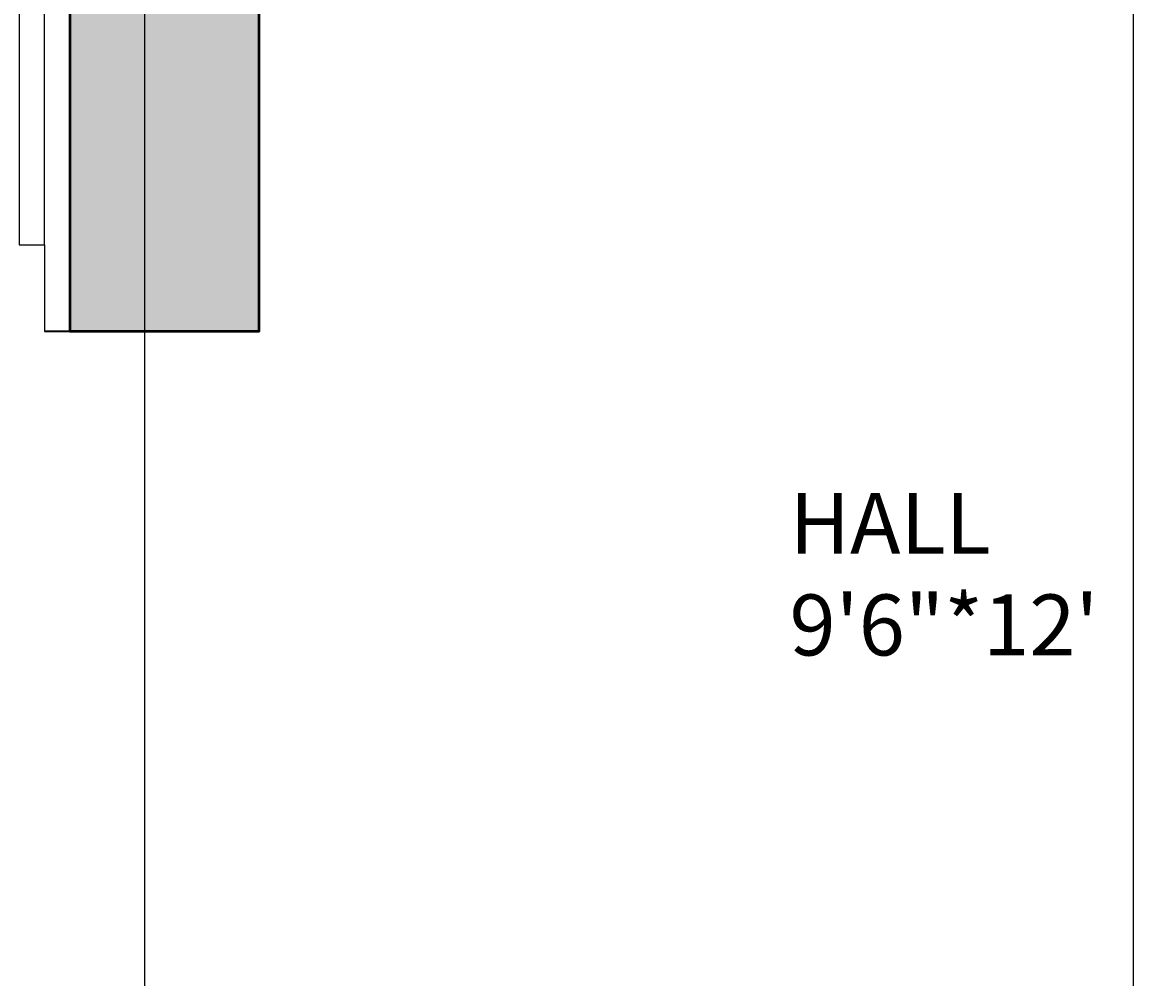
# Model space of a CAD drawing. Units: inches. Extents: x 1998 to 2588, y 1139 to 1977.
# Tile 25 of 134: x 2220 to 2289, y 1427 to 1484. Entities that reach past the tile are written whole.
import ezdxf

# ---------------------------------------------------------------- set-up
doc = ezdxf.new("R2010")
doc.units = ezdxf.units.IN
for name, color, linetype, lineweight in [('A-ANNO-DIMS', 2, 'Continuous', 18), ('A-AREA-IDEN', 7, 'Continuous', 18), ('A-COLS-PATT', 250, 'Continuous', 13), ('COLUMN', 10, 'Continuous', 50), ('DOOR', 52, 'Continuous', 25), ('WALL', 200, 'Continuous', 35)]:
    doc.layers.add(name, color=color, linetype=linetype, lineweight=lineweight)
doc.styles.get("Standard").update_dxf_attribs({"font": 'arial.ttf'})
doc.dimstyles.get("Standard").update_dxf_attribs({"dimtxt": 0.18, "dimasz": 0.18, "dimexe": 0.18, "dimexo": 0.0625, "dimgap": 0.09, "dimtad": 0, "dimtih": 1, "dimtoh": 1, "dimdec": 4, "dimzin": 0, "dimdsep": 46, "dimtxsty": 'Standard', "dimcen": 0.09, "dimadec": 0, "dimazin": 0, "dimtfac": 1, "dimtdec": 4, "dimtofl": 0, "dimtmove": 0, "dimatfit": 3, "dimfxl": 1, "dimtolj": 1, "dimtzin": 0, "dimarcsym": 0})

# ---------------------------------------------------------------- blocks, each defined once
blk = doc.blocks.new('*U2')
for p, q in [((0, 0), (0, -6)), ((40, 0), (40, -6))]:
    blk.add_line(p, q)
blk.add_lwpolyline([(0, 0), (0, 40), (1.75, 40), (1.75, 0)], close=True)
blk.add_arc((0, 0), 40, 0, 90)
blk = doc.blocks.new('*D23')
at = {"layer": 'A-ANNO-DIMS', "color": 0, "lineweight": -2, "transparency": 16777216}
for p, q in [((2549.179, 1476.17), (2549.179, 1138.602)), ((2059.473, 1413.17), (2059.473, 1138.602)), ((2059.653, 1138.782), (2303.928, 1138.782)), ((2548.999, 1138.782), (2304.723, 1138.782))]:
    blk.add_line(p, q, dxfattribs=at)
at = {"layer": 'A-ANNO-DIMS', "color": 0, "transparency": 16777216}
for points in [[(2059.653, 1138.812), (2059.653, 1138.752), (2059.473, 1138.782)], [(2548.999, 1138.812), (2548.999, 1138.752), (2549.179, 1138.782)]]:
    blk.add_solid(points, dxfattribs=at)
at = {"layer": 'Defpoints', "color": 0, "transparency": 16777216}
for p in [(2549.179, 1476.232), (2059.473, 1413.232), (2549.179, 1138.782)]:
    blk.add_point(p, dxfattribs=at)
at = {"layer": 'A-ANNO-DIMS', "color": 0, "transparency": 16777216, "insert": (2304.326, 1138.782), "char_height": 0.18, "attachment_point": 5}
blk.add_mtext('\\A1;489.7', dxfattribs=at)
blk = doc.blocks.new('*D41')
at = {"layer": 'A-ANNO-DIMS', "color": 0, "lineweight": -2, "transparency": 16777216}
for p, q in [((2227.473, 1588.67), (2227.473, 1138.602)), ((2287.473, 1588.67), (2287.473, 1138.602)), ((2227.653, 1138.782), (2257.254, 1138.782)), ((2287.293, 1138.782), (2257.692, 1138.782))]:
    blk.add_line(p, q, dxfattribs=at)
at = {"layer": 'A-ANNO-DIMS', "color": 0, "transparency": 16777216}
for points in [[(2227.653, 1138.812), (2227.653, 1138.752), (2227.473, 1138.782)], [(2287.293, 1138.812), (2287.293, 1138.752), (2287.473, 1138.782)]]:
    blk.add_solid(points, dxfattribs=at)
at = {"layer": 'Defpoints', "color": 0, "transparency": 16777216}
for p in [(2227.473, 1588.732), (2287.473, 1588.732), (2287.473, 1138.782)]:
    blk.add_point(p, dxfattribs=at)
at = {"layer": 'A-ANNO-DIMS', "color": 0, "transparency": 16777216, "insert": (2257.473, 1138.782), "char_height": 0.18, "attachment_point": 5}
blk.add_mtext('\\A1;60', dxfattribs=at)

msp = doc.modelspace()

# ---------------------------------------------------------------- hatches: boundary and pattern name
at = {"layer": 'A-COLS-PATT'}
h = msp.add_hatch(color=256, dxfattribs=at)
h.dxf.hatch_style = 1
h.paths.add_polyline_path([(2099.4125, 1888.7324), (2087.9729, 1888.7324), (2087.9729, 1868.3278), (2099.4125, 1868.3278)])
h.paths.add_polyline_path([(2234.4125, 1888.7324), (2222.9729, 1888.7324), (2222.9729, 1868.3278), (2234.4125, 1868.3278)])
h.paths.add_polyline_path([(2341.4729, 1886.637), (2330.0332, 1886.637), (2330.0332, 1866.2324), (2341.4729, 1866.2324)])
h.paths.add_polyline_path([(2507.8006, 1882.7324), (2487.396, 1882.7324), (2487.396, 1871.2927), (2507.8006, 1871.2927)])
h.paths.add_polyline_path([(2510.9729, 1766.672), (2490.5682, 1766.672), (2490.5682, 1755.2324), (2510.9729, 1755.2324)])
h.paths.add_polyline_path([(2345.9729, 1759.7324), (2334.5332, 1759.7324), (2334.5332, 1739.3278), (2345.9729, 1739.3278)])
h.paths.add_polyline_path([(2234.4125, 1774.3318), (2222.9729, 1774.3318), (2222.9729, 1753.9272), (2234.4125, 1753.9272)])
h.paths.add_polyline_path([(2099.4125, 1775.637), (2087.9729, 1775.637), (2087.9729, 1755.2324), (2099.4125, 1755.2324)])
h.paths.add_polyline_path([(2098.0956, 1593.7241), (2077.691, 1593.7241), (2077.691, 1582.2845), (2098.0956, 1582.2845)])
h.paths.add_polyline_path([(2227.4729, 1604.637), (2216.0332, 1604.637), (2216.0332, 1584.2324), (2227.4729, 1584.2324)])
h.paths.add_polyline_path([(2345.9729, 1647.5211), (2334.5332, 1647.5211), (2334.5332, 1627.1165), (2345.9729, 1627.1165)])
h.paths.add_polyline_path([(2522.3775, 1641.2324), (2501.9729, 1641.2324), (2501.9729, 1629.7927), (2522.3775, 1629.7927)])
h.paths.add_polyline_path([(2522.3775, 1480.7324), (2501.9729, 1480.7324), (2501.9729, 1469.2927), (2522.3775, 1469.2927)])
h.paths.add_polyline_path([(2345.9729, 1488.5616), (2334.5332, 1488.5616), (2334.5332, 1468.1569), (2345.9729, 1468.1569)])
h.paths.add_polyline_path([(2234.4125, 1486.137), (2227.4729, 1486.137), (2227.4729, 1465.7324), (2234.4125, 1465.7324)])
h.paths.add_polyline_path([(2227.4729, 1486.137), (2222.9729, 1486.137), (2222.9729, 1465.7324), (2227.4729, 1465.7324)])
h.paths.add_polyline_path([(2108.3775, 1470.2324), (2087.9729, 1470.2324), (2087.9729, 1458.7927), (2108.3775, 1458.7927)])
h.paths.add_polyline_path([(2096.9729, 1365.5012), (2087.9729, 1365.5012), (2087.9729, 1345.0966), (2096.9729, 1345.0966)])
h.paths.add_polyline_path([(2087.9729, 1365.5012), (2085.5332, 1365.5012), (2085.5332, 1345.0966), (2087.9729, 1345.0966)])
h.paths.add_polyline_path([(2234.4125, 1285.137), (2222.9729, 1285.137), (2222.9729, 1264.7324), (2234.4125, 1264.7324)])
h.paths.add_polyline_path([(2345.9729, 1285.137), (2334.5332, 1285.137), (2334.5332, 1264.7324), (2345.9729, 1264.7324)])
h.paths.add_polyline_path([(2503.1458, 1240.172), (2482.7412, 1240.172), (2482.7412, 1228.7324), (2503.1458, 1228.7324)])
h.paths.add_polyline_path([(2510.9729, 1369.172), (2490.5682, 1369.172), (2490.5682, 1357.7324), (2510.9729, 1357.7324)])

# ---------------------------------------------------------------- linework, layer by layer
at = {"layer": 'COLUMN'}
msp.add_lwpolyline([(2222.9729, 1486.137), (2234.4125, 1486.137), (2234.4125, 1465.7324), (2222.9729, 1465.7324)], close=True, dxfattribs=at)
at = {"layer": 'WALL'}
msp.add_line((2227.4729, 1465.7324), (2221.4126, 1465.7324), dxfattribs=at)

# ---------------------------------------------------------------- block references
at = {"layer": 'DOOR', "xscale": -0.877957807115804, "yscale": 0.877957807115804, "zscale": 0.877957807115804}
msp.add_blockref('*U2', (2221.4126, 1471.0001), dxfattribs=at)

# ---------------------------------------------------------------- texts
at = {"layer": 'A-AREA-IDEN', "insert": (2266.6247, 1455.9484), "char_height": 3.69875, "attachment_point": 1}
msp.add_mtext_dynamic_manual_height_columns('HALL\\P9\'6"*12\'', width=110.572713, gutter_width=18.4938, heights=[0], dxfattribs=at)

# ---------------------------------------------------------------- dimensions: what is measured, and where the dimension line sits
at = {"layer": 'A-ANNO-DIMS'}
for base, p1, p2, override, picture, middle in [((2287.4729, 1138.7824), (2227.4729, 1588.7324), (2287.4729, 1588.7324), {"dimdec": 0, "dimlfac": 1, "dimrnd": 0, "dimzin": 0, "dimdsep": 46, "dimlunit": 2}, '*D41', (2257.4729, 1138.7824)), ((2549.1786, 1138.7824), (2059.4729, 1413.2324), (2549.1786, 1476.2324), {"dimdec": 1, "dimlfac": 1, "dimrnd": 0, "dimzin": 0, "dimdsep": 46, "dimlunit": 2}, '*D23', (2304.3257, 1138.7824))]:
    dim = msp.add_linear_dim(base=base, p1=p1, p2=p2, dimstyle='Standard', override=override, dxfattribs=at)
    dim.commit()
    dim.dimension.update_dxf_attribs({"geometry": picture, "text_midpoint": middle})

doc.saveas('drawing.dxf')
